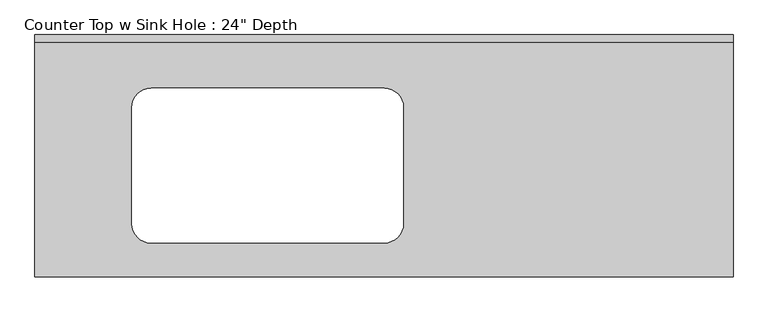
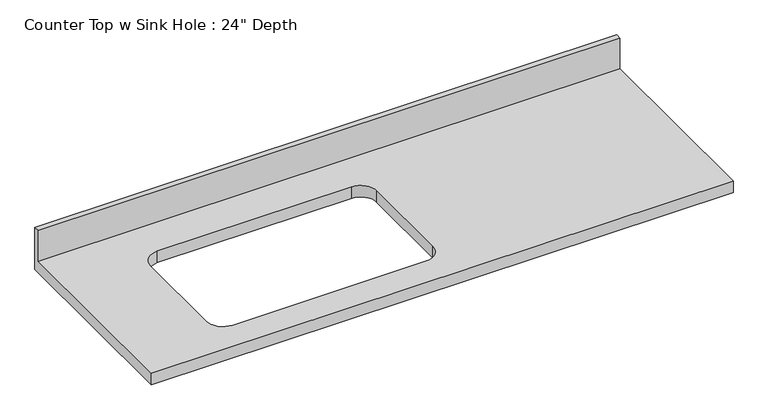
"""IFC4 building model written with IfcOpenShell, lengths in millimetres: furniture geometry."""

from ifc_helpers import new_model, si_unit, frame, origin, place, context, project, spatial, polyline, circle_curve, source, transform, mapped, element, save
from ifc_brep_helpers import plane_surface, revolved_surface, advanced_brep


def furniture_1447f48d(model_context):
    return source(origin(), model_context, "Body", "AdvancedBrep", [
        advanced_brep(
        [(-1200.4622951, -635.0, 914.4), (628.3377049, -635.0, 914.4), (628.3377049, -19.05, 914.4), (-1200.4622951, -19.05, 914.4), (-895.6622951, -139.7, 914.4), (-286.0622951, -139.7, 914.4), (-235.2622951, -190.5, 914.4), (-235.2622951, -495.3, 914.4), (-286.0622951, -546.1, 914.4), (-895.6622951, -546.1, 914.4), (-946.4622951, -495.3, 914.4), (-946.4622951, -190.5, 914.4), (628.3377049, 0.0, 876.3), (628.3377049, -635.0, 876.3), (-1200.4622951, -635.0, 876.3), (-1200.4622951, 0.0, 876.3), (-286.0622951, -139.7, 876.3), (-895.6622951, -139.7, 876.3), (-946.4622951, -190.5, 876.3), (-946.4622951, -495.3, 876.3), (-895.6622951, -546.1, 876.3), (-286.0622951, -546.1, 876.3), (-235.2622951, -495.3, 876.3), (-235.2622951, -190.5, 876.3), (-1200.4622951, 0.0, 1016.0), (628.3377049, 0.0, 1016.0), (-1200.4622951, -19.05, 1016.0), (628.3377049, -19.05, 1016.0)],
        [
            (0, 1),
            (1, 2),
            (2, 3),
            (3, 0),
            (4, 5),
            (5, 6, circle_curve(frame((-286.0622951, -190.5, 914.4), z_axis=(0.0, 0.0, -1.0), x_axis=(1.0, 0.0, 0.0)), 50.8)),
            (6, 7),
            (7, 8, circle_curve(frame((-286.0622951, -495.3, 914.4), z_axis=(0.0, 0.0, -1.0), x_axis=(1.0, 0.0, 0.0)), 50.8)),
            (8, 9),
            (9, 10, circle_curve(frame((-895.6622951, -495.3, 914.4), z_axis=(0.0, 0.0, -1.0), x_axis=(1.0, 0.0, 0.0)), 50.8)),
            (10, 11),
            (11, 4, circle_curve(frame((-895.6622951, -190.5, 914.4), z_axis=(0.0, 0.0, -1.0), x_axis=(1.0, 0.0, 0.0)), 50.8)),
            (12, 13),
            (13, 14),
            (14, 15),
            (15, 12),
            (16, 17),
            (17, 18, circle_curve(frame((-895.6622951, -190.5, 876.3), z_axis=(0.0, 0.0, 1.0), x_axis=(1.0, 0.0, 0.0)), 50.8)),
            (18, 19),
            (19, 20, circle_curve(frame((-895.6622951, -495.3, 876.3), z_axis=(0.0, 0.0, 1.0), x_axis=(1.0, 0.0, 0.0)), 50.8)),
            (20, 21),
            (21, 22, circle_curve(frame((-286.0622951, -495.3, 876.3), z_axis=(0.0, 0.0, 1.0), x_axis=(1.0, 0.0, 0.0)), 50.8)),
            (22, 23),
            (23, 16, circle_curve(frame((-286.0622951, -190.5, 876.3), z_axis=(0.0, 0.0, 1.0), x_axis=(1.0, 0.0, 0.0)), 50.8)),
            (15, 24),
            (24, 25),
            (25, 12),
            (14, 0),
            (3, 26),
            (26, 24),
            (13, 1),
            (25, 27),
            (27, 2),
            (4, 17),
            (16, 5),
            (11, 18),
            (10, 19),
            (9, 20),
            (8, 21),
            (7, 22),
            (6, 23),
            (26, 27),
        ],
        [
            plane_surface(frame((-1200.4622951, 0.0, 914.4), z_axis=(0.0, 0.0, 1.0), x_axis=(-1.0, 0.0, 0.0))),
            plane_surface(frame((-1200.4622951, 0.0, 876.3), z_axis=(0.0, 0.0, -1.0), x_axis=(1.0, 0.0, 0.0))),
            plane_surface(frame((628.3377049, 0.0, 914.4), z_axis=(0.0, 1.0, 0.0), x_axis=(0.0, 0.0, -1.0))),
            plane_surface(frame((-1200.4622951, 0.0, 914.4), z_axis=(-1.0, 0.0, 0.0), x_axis=(0.0, 0.0, -1.0))),
            plane_surface(frame((-1200.4622951, -635.0, 914.4), z_axis=(0.0, -1.0, 0.0), x_axis=(0.0, 0.0, -1.0))),
            plane_surface(frame((628.3377049, -635.0, 914.4), z_axis=(1.0, 0.0, 0.0), x_axis=(0.0, 0.0, -1.0))),
            plane_surface(frame((-286.0622951, -139.7, 914.4), z_axis=(0.0, -1.0, 0.0), x_axis=(0.0, 0.0, -1.0))),
            revolved_surface(polyline([(-844.8622951000001, -190.5, 914.4), (-844.8622951000001, -190.5, 876.3)]), (-895.6622951, -190.5, 876.3), (0.0, 0.0, 1.0)),
            plane_surface(frame((-946.4622951, -190.5, 914.4), z_axis=(1.0, 0.0, 0.0), x_axis=(0.0, 0.0, -1.0))),
            revolved_surface(polyline([(-844.8622951000001, -495.3, 914.4), (-844.8622951000001, -495.3, 876.3)]), (-895.6622951, -495.3, 876.3), (0.0, 0.0, 1.0)),
            plane_surface(frame((-895.6622951, -546.1, 914.4), z_axis=(0.0, 1.0, 0.0), x_axis=(0.0, 0.0, -1.0))),
            revolved_surface(polyline([(-235.26229509999996, -495.3, 914.4), (-235.26229509999996, -495.3, 876.3)]), (-286.0622951, -495.3, 876.3), (0.0, 0.0, 1.0)),
            plane_surface(frame((-235.2622951, -495.3, 914.4), z_axis=(-1.0, 0.0, 0.0), x_axis=(0.0, 0.0, -1.0))),
            revolved_surface(polyline([(-235.26229509999996, -190.5, 914.4), (-235.26229509999996, -190.5, 876.3)]), (-286.0622951, -190.5, 876.3), (0.0, 0.0, 1.0)),
            plane_surface(frame((-1200.4622951, 0.0, 1016.0), z_axis=(0.0, 0.0, 1.0), x_axis=(0.0, -1.0, 0.0))),
            plane_surface(frame((-1200.4622951, -19.05, 1016.0), z_axis=(0.0, -1.0, 0.0), x_axis=(0.0, 0.0, -1.0))),
        ],
        [
            (0, [[1, 2, 3, 4], [5, 6, 7, 8, 9, 10, 11, 12]]),
            (1, [[13, 14, 15, 16], [17, 18, 19, 20, 21, 22, 23, 24]]),
            (2, [[-16, 25, 26, 27]]),
            (3, [[-15, 28, -4, 29, 30, -25]]),
            (4, [[-1, -28, -14, 31]]),
            (5, [[-13, -27, 32, 33, -2, -31]]),
            (6, [[34, -17, 35, -5]]),
            (7, [[-34, -12, 36, -18]]),
            (8, [[-36, -11, 37, -19]]),
            (9, [[-37, -10, 38, -20]]),
            (10, [[-38, -9, 39, -21]]),
            (11, [[-39, -8, 40, -22]]),
            (12, [[-40, -7, 41, -23]]),
            (13, [[-35, -24, -41, -6]]),
            (14, [[-30, 42, -32, -26]]),
            (15, [[-42, -29, -3, -33]]),
        ],
    ),
    ])


if __name__ == "__main__":
    model = new_model("IFC4")
    model_context = context("Model", 3, world=origin())
    ifc_project = project(units=[si_unit("LENGTHUNIT", "METRE", prefix="MILLI")], contexts=[model_context])
    site = spatial("IfcSite", under=ifc_project)
    building = spatial("IfcBuilding", under=site)
    placement = place(None, origin())
    furniture_shape = furniture_1447f48d(model_context)
    element("IfcFurniture", 1, ObjectType="Counter Top w Sink Hole : 24\" Depth", at=placement, inside=building, context=model_context, shape_type="MappedRepresentation", body=[
        mapped(furniture_shape, transform((0.0, 0.0, 0.0), x_axis=(1.0, 0.0, 0.0), y_axis=(0.0, 1.0, 0.0), z_axis=(0.0, 0.0, 1.0))),
    ])
    save(model, "model.ifc")

# Revit data of these elements
# Type "Counter Top w Sink Hole : 24\" Depth"
#   Assembly Code = "C1030400"
#   Counter Thickness = 0' - 1 1/2"
#   Depth = 2' - 1"
#   Height = 3' - 0"
#   Length [instance default] = 8' - 0"
#   Sink Location [instance default] = 2' - 0"
#   Sink Location To Wall [instance default] = 0' - 6"
#   Sink Opening Depth [instance default] = 1' - 3"
#   Sink Opening Width [instance default] = 2' - 3"
#   Counter Top Material = none
#   Default Elevation = 0
# Element 1 (IfcFurniture, "Counter Top w Sink Hole : 24\" Depth")
#   Length = 6' - 0"
#   Materials on its faces: "Counter Top"
# Materials
#   "Counter Top": class "Wood", colour RGB 226 177 128, transparency 0
